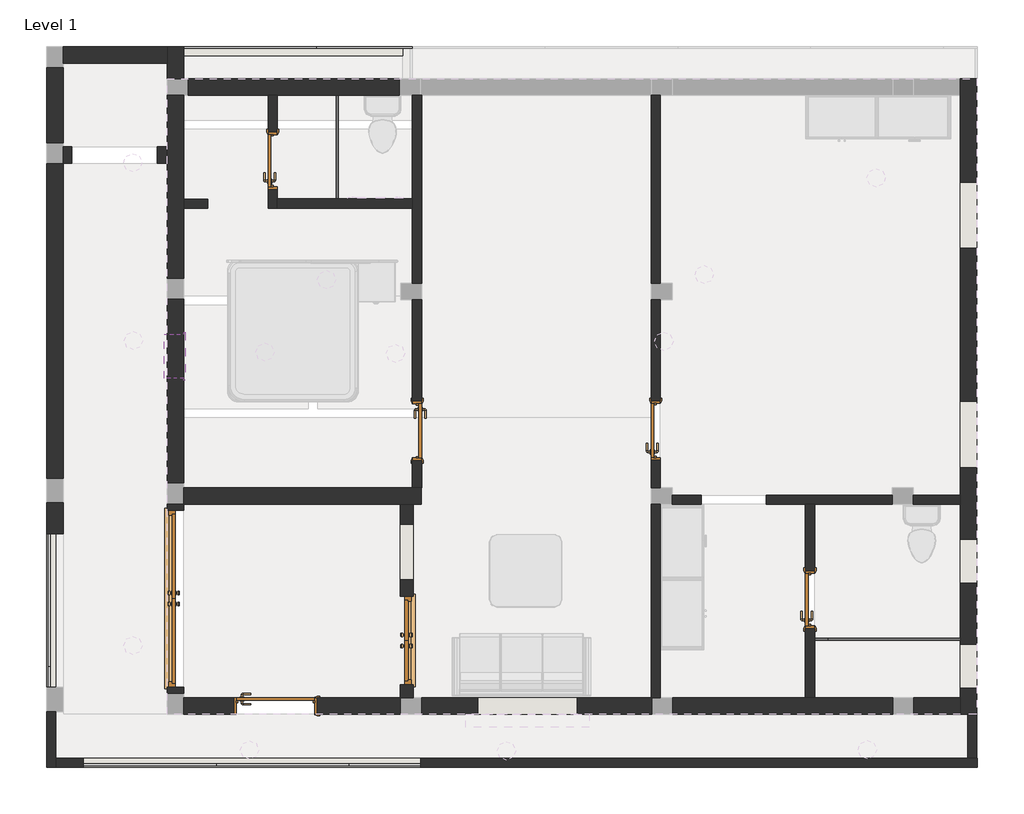
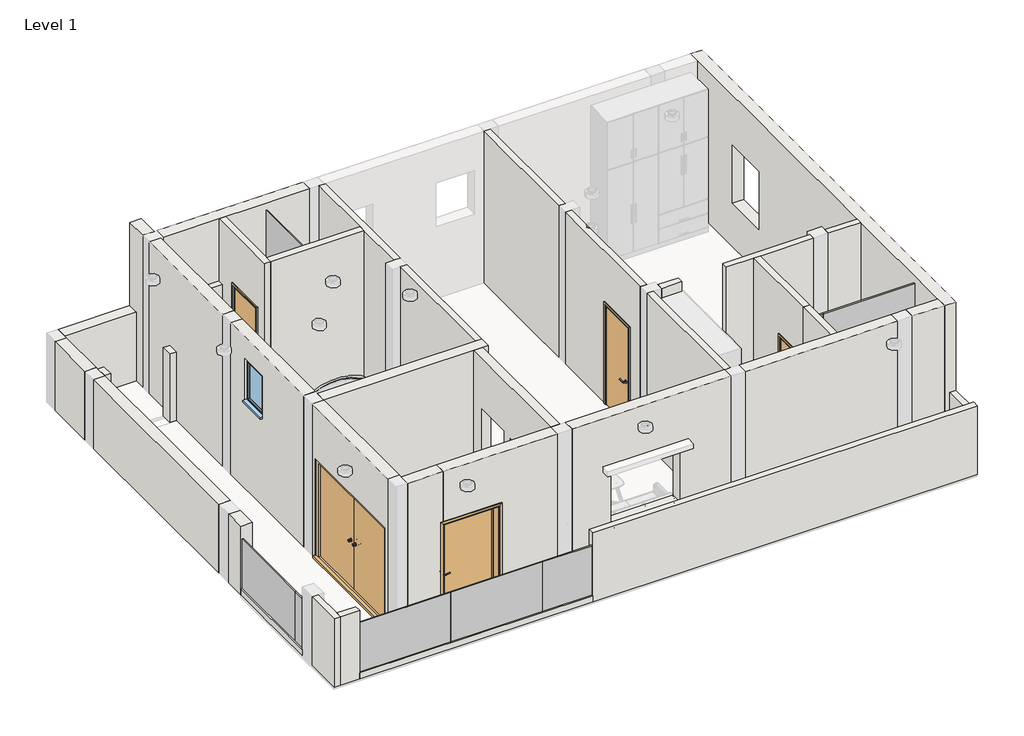
# One storey, part 1 of 2: 39 walls, 10 plates, 7 doors, 1 window.
"""IFC4 building model written with IfcOpenShell, lengths in millimetres."""

from ifc_helpers import new_model, si_unit, frame, origin, place, context, project, spatial, polyline, outline, extrude, faceted_brep, transform, mapped, element, save
from components import doors_extdbl_flush_md_0ef74d11, doors_extdbl_flush_md_2_f65acf09, doors_intsgl_d3_a25f8c6e, doors_intsgl_d4_4271d8f6, doors_intsgl_d2_d6dd0e7a, system_panel_glazed_6338a664, system_panel_glazed_e6893c60, system_panel_glazed_6661c6ea, system_panel_glazed_2d3c21f4, system_panel_glazed_3dcdd35b, system_panel_glazed_bdd68f76, system_panel_glazed_6933bc29, system_panel_glazed_1575378d, windows_sgl_plain_610x910mm_8d1346b0

model = new_model("IFC4")

# Units and contexts
model_context = context("Model", 3, world=origin())
ifc_project = project(units=[si_unit("LENGTHUNIT", "METRE", prefix="MILLI")], contexts=[model_context])

# Site, building, storey
site = spatial("IfcSite", under=ifc_project)
building = spatial("IfcBuilding", under=site)
storey = spatial("IfcBuildingStorey", under=building, Name="Level 1", Elevation=3200.4)

# Doors
placement = place(None, origin())
doors_extdbl_flush_md_shape = doors_extdbl_flush_md_0ef74d11(model_context)
element("IfcDoor", 1, ObjectType="Doors_ExtDbl_Flush : MD", at=placement, inside=storey, context=model_context, shape_type="MappedRepresentation", body=[
    mapped(doors_extdbl_flush_md_shape, transform((-11061.4858712, -2060.9296054, 3200.4), x_axis=(0.0, 1.0, 0.0), y_axis=(-1.0, 0.0, 0.0), z_axis=(0.0, 0.0, 1.0))),
])
doors_extdbl_flush_md_2_shape = doors_extdbl_flush_md_2_f65acf09(model_context)
element("IfcDoor", 2, ObjectType="Doors_ExtDbl_Flush : MD 2", at=placement, inside=storey, context=model_context, shape_type="MappedRepresentation", body=[
    mapped(doors_extdbl_flush_md_2_shape, transform((-7871.4445565, -2638.7796054, 3200.4), x_axis=(0.0, -1.0, 0.0), y_axis=(1.0, 0.0, 0.0), z_axis=(0.0, 0.0, 1.0))),
])
doors_intsgl_d3_shape = doors_intsgl_d3_a25f8c6e(model_context)
element("IfcDoor", 3, ObjectType="Doors_IntSgl : D3", at=placement, inside=storey, context=model_context, shape_type="MappedRepresentation", body=[
    mapped(doors_intsgl_d3_shape, transform((-2315.0983223, -2074.5629976, 3200.4), x_axis=(0.0, 1.0, 0.0), y_axis=(-1.0, 0.0, 0.0), z_axis=(0.0, 0.0, 1.0))),
])
element("IfcDoor", 4, ObjectType="Doors_IntSgl : D3", at=placement, inside=storey, context=model_context, shape_type="MappedRepresentation", body=[
    mapped(doors_intsgl_d3_shape, transform((-9717.6156351, 3973.7139975, 3200.4), x_axis=(0.0, 1.0, 0.0), y_axis=(-1.0, 0.0, 0.0), z_axis=(0.0, 0.0, 1.0))),
])
doors_intsgl_d4_shape = doors_intsgl_d4_4271d8f6(model_context)
element("IfcDoor", 5, ObjectType="Doors_IntSgl : D4", at=placement, inside=storey, context=model_context, shape_type="MappedRepresentation", body=[
    mapped(doors_intsgl_d4_shape, transform((-4442.6060272, 254.9952475, 3200.4), x_axis=(0.0, 1.0, 0.0), y_axis=(-1.0, 0.0, 0.0), z_axis=(0.0, 0.0, 1.0))),
])
element("IfcDoor", 6, ObjectType="Doors_IntSgl : D4", at=placement, inside=storey, context=model_context, shape_type="MappedRepresentation", body=[
    mapped(doors_intsgl_d4_shape, transform((-7729.6634981, 250.4703946, 3200.4), x_axis=(0.0, -1.0, 0.0), y_axis=(1.0, 0.0, 0.0), z_axis=(0.0, 0.0, 1.0))),
])
doors_intsgl_d2_shape = doors_intsgl_d2_d6dd0e7a(model_context)
element("IfcDoor", 7, ObjectType="Doors_IntSgl : d2", at=placement, inside=storey, context=model_context, shape_type="MappedRepresentation", body=[
    mapped(doors_intsgl_d2_shape, transform((-9681.1945565, -3540.4796054, 3200.4), x_axis=(1.0, 0.0, 0.0), y_axis=(0.0, 1.0, 0.0), z_axis=(0.0, 0.0, 1.0))),
])

# Plates
system_panel_glazed_shape = system_panel_glazed_6338a664(model_context)
element("IfcPlate", 8, ObjectType="System Panel : Glazed", at=placement, inside=storey, context=model_context, shape_type="MappedRepresentation", body=[
    mapped(system_panel_glazed_shape, transform((-10032.185871, 5496.5824405, 3200.4), x_axis=(1.0, 0.0, 0.0), y_axis=(0.0, 1.0, 0.0), z_axis=(0.0, 0.0, 1.0))),
])
system_panel_glazed_2_shape = system_panel_glazed_e6893c60(model_context)
element("IfcPlate", 9, ObjectType="System Panel : Glazed", at=placement, inside=storey, context=model_context, shape_type="MappedRepresentation", body=[
    mapped(system_panel_glazed_2_shape, transform((-8458.035871, 5496.5824405, 3200.4), x_axis=(1.0, 0.0, 0.0), y_axis=(0.0, 1.0, 0.0), z_axis=(0.0, 0.0, 1.0))),
])
system_panel_glazed_3_shape = system_panel_glazed_6661c6ea(model_context)
element("IfcPlate", 10, ObjectType="System Panel : Glazed", at=placement, inside=storey, context=model_context, shape_type="MappedRepresentation", body=[
    mapped(system_panel_glazed_3_shape, transform((-1157.4352301, -2582.5629976, 3200.4), x_axis=(-1.0, 0.0, 0.0), y_axis=(0.0, -1.0, 0.0), z_axis=(0.0, 0.0, 1.0))),
])
system_panel_glazed_4_shape = system_panel_glazed_2d3c21f4(model_context)
element("IfcPlate", 11, ObjectType="System Panel : Glazed", at=placement, inside=storey, context=model_context, shape_type="MappedRepresentation", body=[
    mapped(system_panel_glazed_4_shape, transform((-2162.0167763, -2582.5629976, 3200.4), x_axis=(-1.0, 0.0, 0.0), y_axis=(0.0, -1.0, 0.0), z_axis=(0.0, 0.0, 1.0))),
])
system_panel_glazed_5_shape = system_panel_glazed_3dcdd35b(model_context)
element("IfcPlate", 12, ObjectType="System Panel : Glazed", at=placement, inside=storey, context=model_context, shape_type="MappedRepresentation", body=[
    mapped(system_panel_glazed_5_shape, transform((-12836.0604224, -2082.0550561, 3327.4), x_axis=(0.0, -1.0, 0.0), y_axis=(1.0, 0.0, 0.0), z_axis=(0.0, 0.0, 1.0))),
])
element("IfcPlate", 13, ObjectType="System Panel : Glazed", at=placement, inside=storey, context=model_context, shape_type="MappedRepresentation", body=[
    mapped(system_panel_glazed_5_shape, transform((-11413.0604222, -4385.9896501, 3327.4), x_axis=(1.0, 0.0, 0.0), y_axis=(0.0, 1.0, 0.0), z_axis=(0.0, 0.0, 1.0))),
])
element("IfcPlate", 14, ObjectType="System Panel : Glazed", at=placement, inside=storey, context=model_context, shape_type="MappedRepresentation", body=[
    mapped(system_panel_glazed_5_shape, transform((-9583.060422, -4385.9896501, 3327.4), x_axis=(1.0, 0.0, 0.0), y_axis=(0.0, 1.0, 0.0), z_axis=(0.0, 0.0, 1.0))),
])
system_panel_glazed_6_shape = system_panel_glazed_bdd68f76(model_context)
element("IfcPlate", 15, ObjectType="System Panel : Glazed", at=placement, inside=storey, context=model_context, shape_type="MappedRepresentation", body=[
    mapped(system_panel_glazed_6_shape, transform((-8173.172826, -4385.9896501, 3327.4), x_axis=(1.0, 0.0, 0.0), y_axis=(0.0, 1.0, 0.0), z_axis=(0.0, 0.0, 1.0))),
])
system_panel_glazed_7_shape = system_panel_glazed_6933bc29(model_context)
element("IfcPlate", 16, ObjectType="System Panel : Glazed", at=placement, inside=storey, context=model_context, shape_type="MappedRepresentation", body=[
    mapped(system_panel_glazed_7_shape, transform((-12836.0604224, -3139.0723532, 3327.4), x_axis=(0.0, -1.0, 0.0), y_axis=(1.0, 0.0, 0.0), z_axis=(0.0, 0.0, 1.0))),
])
system_panel_glazed_8_shape = system_panel_glazed_1575378d(model_context)
element("IfcPlate", 17, ObjectType="System Panel : Glazed", at=placement, inside=storey, context=model_context, shape_type="MappedRepresentation", body=[
    mapped(system_panel_glazed_8_shape, transform((-8866.3134981, 4161.7783231, 3200.4), x_axis=(0.0, -1.0, 0.0), y_axis=(1.0, 0.0, 0.0), z_axis=(0.0, 0.0, 1.0))),
])

# Walls
element("IfcWall", 18, ObjectType="5\"", at=placement, inside=storey, context=model_context, shape_type="Brep", body=[
    faceted_brep([(-7926.5134981, 5546.4824405, 3200.4), (-10947.1858712, 5546.4824405, 3200.4), (-10947.1858712, 5546.4824405, 3276.6), (-7926.5134981, 5546.4824405, 3276.6), (-7926.5134981, 5419.4824405, 3200.4), (-7926.5134981, 5419.4824405, 3276.6), (-10947.1858712, 5419.4824405, 3276.6), (-10947.1858712, 5419.4824405, 3200.4), (-10947.1858712, 5545.7949405, 3200.4)], [[[0, 1, 2, 3]], [[4, 5, 6, 7]], [[1, 0, 4, 7, 8]], [[2, 1, 8, 7, 6]], [[3, 2, 6, 5]], [[0, 3, 5, 4]]]),
])
element("IfcWall", 19, ObjectType="5\"", at=placement, inside=storey, context=model_context, shape_type="Brep", body=[
    faceted_brep([(-12836.0604224, -3623.9896501, 3200.4), (-12836.0604224, -4385.9896501, 3200.4), (-12836.0604224, -4385.9896501, 4648.2), (-12836.0604224, -3623.9896501, 4648.2), (-12709.0604224, -3623.9896501, 3200.4), (-12709.0604224, -3623.9896501, 4648.2), (-12709.0604224, -4258.9896501, 4648.2), (-12709.0604224, -4385.9896501, 4648.2), (-12709.0604224, -4385.9896501, 3200.4), (-12709.0604224, -4258.9896501, 3200.4)], [[[0, 1, 2, 3]], [[4, 5, 6, 7, 8, 9]], [[1, 0, 4, 9, 8]], [[2, 1, 8, 7]], [[3, 2, 7, 6, 5]], [[0, 3, 5, 4]]]),
])
element("IfcWall", 20, ObjectType="5\"", at=placement, inside=storey, context=model_context, shape_type="Brep", body=[
    faceted_brep([(-12709.0604224, -4385.9896501, 3200.4), (-12328.0604224, -4385.9896501, 3200.4), (-12328.0604224, -4385.9896501, 3327.4), (-12328.0604224, -4385.9896501, 4648.2), (-12709.0604224, -4385.9896501, 4648.2), (-12709.0604224, -4258.9896501, 3200.4), (-12709.0604224, -4258.9896501, 4648.2), (-12328.0604224, -4258.9896501, 4648.2), (-12328.0604224, -4258.9896501, 3327.4), (-12328.0604224, -4258.9896501, 3200.4)], [[[0, 1, 2, 3, 4]], [[5, 6, 7, 8, 9]], [[1, 0, 5, 9]], [[3, 2, 1, 9, 8, 7]], [[4, 3, 7, 6]], [[0, 4, 6, 5]]]),
])
element("IfcWall", 21, ObjectType="5\"", at=placement, inside=storey, context=model_context, shape_type="Brep", body=[
    faceted_brep([(-7678.28523, -4385.9896501, 3200.4), (-7.48523, -4385.9896501, 3200.4), (-7.48523, -4385.9896501, 4648.2), (-7678.28523, -4385.9896501, 4648.2), (-7678.28523, -4385.9896501, 3327.4), (-7678.28523, -4258.9896501, 3200.4), (-7678.28523, -4258.9896501, 3327.4), (-7678.28523, -4258.9896501, 4648.2), (-7.48523, -4258.9896501, 4648.2), (-7.48523, -4258.9896501, 3200.4), (-13.83523, -4258.9896501, 3200.4), (-140.83523, -4258.9896501, 3200.4)], [[[0, 1, 2, 3, 4]], [[5, 6, 7, 8, 9, 10, 11]], [[1, 0, 5, 11, 10, 9]], [[2, 1, 9, 8]], [[3, 2, 8, 7]], [[0, 4, 3, 7, 6, 5]]]),
])
element("IfcWall", 22, ObjectType="5\"", at=placement, inside=storey, context=model_context, shape_type="SweptSolid", body=[
    extrude(outline(polyline([(-13.83523, -3654.7796054), (-13.83523, -4258.9896501), (-140.83523, -4258.9896501), (-140.83523, -3654.7796054), (-13.83523, -3654.7796054)])), frame((0.0, 0.0, 3200.4), z_axis=(0.0, 0.0, 1.0), x_axis=(1.0, 0.0, 0.0)), (0.0, 0.0, 1.0), 1333.7357837),
])
element("IfcWall", 23, ObjectType="5\"", at=placement, inside=storey, context=model_context, shape_type="SweptSolid", body=[
    extrude(outline(polyline([(-12836.0604224, -3281.0896501), (-12836.0604224, -1167.055056), (-12709.0604224, -1167.055056), (-12709.0604224, -3281.0896501), (-12836.0604224, -3281.0896501)])), frame((0.0, 0.0, 3200.4), z_axis=(0.0, 0.0, 1.0), x_axis=(1.0, 0.0, 0.0)), (0.0, 0.0, 1.0), 127.0),
])
element("IfcWall", 24, ObjectType="5\"", at=placement, inside=storey, context=model_context, shape_type="SweptSolid", body=[
    extrude(outline(polyline([(-7678.28523, -4385.9896501), (-12328.0604224, -4385.9896501), (-12328.0604224, -4258.9896501), (-7678.28523, -4258.9896501), (-7678.28523, -4385.9896501)])), frame((0.0, 0.0, 3200.4), z_axis=(0.0, 0.0, 1.0), x_axis=(1.0, 0.0, 0.0)), (0.0, 0.0, 1.0), 127.0),
])
element("IfcWall", 25, ObjectType="7\"", at=placement, inside=storey, context=model_context, shape_type="SweptSolid", body=[
    extrude(outline(polyline([(-3248.3796054, 5310.4), (-3248.3796054, 3200.4), (-3426.1796054, 3200.4), (-3426.1796054, 6400.8), (-759.1796054, 6400.8), (-759.1796054, 3200.4), (-2029.1796054, 3200.4), (-2029.1796054, 5310.4), (-3248.3796054, 5310.4)]), holes=[polyline([(-1038.5796054, 5334.0), (-1800.5796054, 5334.0), (-1800.5796054, 4114.8), (-1038.5796054, 4114.8), (-1038.5796054, 5334.0)])]), frame((-7960.3445565, 0.0, 0.0), z_axis=(1.0, 0.0, 0.0), x_axis=(0.0, 1.0, 0.0)), (0.0, 0.0, 1.0), 177.8),
])
element("IfcWall", 26, ObjectType="9\"", at=placement, inside=storey, context=model_context, shape_type="SweptSolid", body=[
    extrude(outline(polyline([(-12836.0604224, 4222.4988089), (-12836.0604224, 5253.6949405), (-12607.4604224, 5253.6949405), (-12607.4604224, 4222.4988089), (-12836.0604224, 4222.4988089)])), frame((0.0, 0.0, 3200.4), z_axis=(0.0, 0.0, 1.0), x_axis=(1.0, 0.0, 0.0)), (0.0, 0.0, 1.0), 1447.8),
])
element("IfcWall", 27, ObjectType="9\"", at=placement, inside=storey, context=model_context, shape_type="SweptSolid", body=[
    extrude(outline(polyline([(-12836.0604224, -404.5396501), (-12836.0604224, 3930.3988089), (-12607.4604224, 3930.3988089), (-12607.4604224, -404.5396501), (-12836.0604224, -404.5396501)])), frame((0.0, 0.0, 3200.4), z_axis=(0.0, 0.0, 1.0), x_axis=(1.0, 0.0, 0.0)), (0.0, 0.0, 1.0), 1447.8),
])
element("IfcWall", 28, ObjectType="9\"", at=placement, inside=storey, context=model_context, shape_type="Brep", body=[
    faceted_brep([(-12836.0604224, -743.5406999, 3200.4), (-12836.0604224, -747.4396501, 3200.4), (-12836.0604224, -1167.055056, 3200.4), (-12836.0604224, -1167.055056, 4648.2), (-12836.0604224, -743.5406999, 4648.2), (-12607.4604224, -743.5406999, 3200.4), (-12607.4604224, -743.5406999, 4648.2), (-12607.4604224, -1167.055056, 4648.2), (-12607.4604224, -1167.055056, 3200.4), (-12607.4604224, -747.4396501, 3200.4)], [[[0, 1, 2, 3, 4]], [[5, 6, 7, 8, 9]], [[2, 1, 0, 5, 9, 8]], [[3, 2, 8, 7]], [[4, 3, 7, 6]], [[0, 4, 6, 5]]]),
])
element("IfcWall", 29, ObjectType="9\"", at=placement, inside=storey, context=model_context, shape_type="SweptSolid", body=[
    extrude(outline(polyline([(6400.8, -10240.7910021), (6400.8, -10947.1858712), (3200.4, -10947.1858712), (3200.4, -10259.0445565), (5310.4, -10259.0445565), (5310.4, -10240.7910021), (6400.8, -10240.7910021)])), frame((0.0, -3654.7796054, 0.0), z_axis=(0.0, 1.0, 0.0), x_axis=(0.0, 0.0, 1.0)), (0.0, 0.0, 1.0), 228.6),
])
element("IfcWall", 30, ObjectType="9\"", at=placement, inside=storey, context=model_context, shape_type="SweptSolid", body=[
    extrude(outline(polyline([(3200.4, -7960.3445565), (6400.8, -7960.3445565), (6400.8, -10240.7910021), (5310.4, -10240.7910021), (5310.4, -9103.3445565), (3200.4, -9103.3445565), (3200.4, -7960.3445565)])), frame((0.0, -3654.7796054, 0.0), z_axis=(0.0, 1.0, 0.0), x_axis=(0.0, 0.0, 1.0)), (0.0, 0.0, 1.0), 228.6),
])
element("IfcWall", 31, ObjectType="9\"", at=placement, inside=storey, context=model_context, shape_type="SweptSolid", body=[
    extrude(outline(polyline([(3200.4, -7668.2445565), (3200.4, -4496.93523), (6400.8, -4496.93523), (6400.8, -7668.2445565), (3200.4, -7668.2445565)]), holes=[polyline([(5334.0, -6890.88523), (5334.0, -5519.28523), (4114.8, -5519.28523), (4114.8, -6890.88523), (5334.0, -6890.88523)])]), frame((0.0, -3654.7796054, 0.0), z_axis=(0.0, 1.0, 0.0), x_axis=(0.0, 0.0, 1.0)), (0.0, 0.0, 1.0), 228.6),
])
element("IfcWall", 32, ObjectType="9\"", at=placement, inside=storey, context=model_context, shape_type="SweptSolid", body=[
    extrude(outline(polyline([(-1175.88523, -3654.7796054), (-4204.83523, -3654.7796054), (-4204.83523, -3426.1796054), (-1175.88523, -3426.1796054), (-1175.88523, -3654.7796054)])), frame((0.0, 0.0, 3200.4), z_axis=(0.0, 0.0, 1.0), x_axis=(1.0, 0.0, 0.0)), (0.0, 0.0, 1.0), 3200.4),
])
element("IfcWall", 33, ObjectType="9\"", at=placement, inside=storey, context=model_context, shape_type="SweptSolid", body=[
    extrude(outline(polyline([(-242.43523, -3654.7796054), (-883.78523, -3654.7796054), (-883.78523, -3426.1796054), (-242.43523, -3426.1796054), (-242.43523, -3654.7796054)])), frame((0.0, 0.0, 3200.4), z_axis=(0.0, 0.0, 1.0), x_axis=(1.0, 0.0, 0.0)), (0.0, 0.0, 1.0), 3200.4),
])
element("IfcWall", 34, ObjectType="9\"", at=placement, inside=storey, context=model_context, shape_type="Brep", body=[
    faceted_brep([(-13.83523, -3654.7796054, 3200.4), (-13.83523, 5101.6327475, 3200.4), (-13.83523, 5101.6327475, 6400.8), (-13.83523, -3654.7796054, 6400.8), (-13.83523, -3654.7796054, 4534.1357837), (-13.83523, 2764.8327475, 5334.0), (-13.83523, 3679.2327475, 5334.0), (-13.83523, 3679.2327475, 4114.8), (-13.83523, 2764.8327475, 4114.8), (-13.83523, -257.7672525, 5334.0), (-13.83523, 656.6327475, 5334.0), (-13.83523, 656.6327475, 4114.8), (-13.83523, -257.7672525, 4114.8), (-13.83523, -2689.5796054, 4724.4), (-13.83523, -2689.5796054, 4114.8), (-13.83523, -3299.1796054, 4114.8), (-13.83523, -3299.1796054, 4724.4), (-13.83523, -1241.7796054, 4724.4), (-13.83523, -1241.7796054, 4114.8), (-13.83523, -1851.3796054, 4114.8), (-13.83523, -1851.3796054, 4724.4), (-242.43523, -3654.7796054, 3200.4), (-242.43523, -3654.7796054, 6400.8), (-242.43523, -3426.1796054, 6400.8), (-242.43523, 4873.0327475, 6400.8), (-242.43523, 5101.6327475, 6400.8), (-242.43523, 5101.6327475, 3200.4), (-242.43523, 4873.0327475, 3200.4), (-242.43523, -3426.1796054, 3200.4), (-242.43523, 2764.8327475, 5334.0), (-242.43523, 2764.8327475, 4114.8), (-242.43523, 3679.2327475, 4114.8), (-242.43523, 3679.2327475, 5334.0), (-242.43523, -257.7672525, 5334.0), (-242.43523, -257.7672525, 4114.8), (-242.43523, 656.6327475, 4114.8), (-242.43523, 656.6327475, 5334.0), (-242.43523, -2689.5796054, 4724.4), (-242.43523, -3299.1796054, 4724.4), (-242.43523, -3299.1796054, 4114.8), (-242.43523, -2689.5796054, 4114.8), (-242.43523, -1241.7796054, 4724.4), (-242.43523, -1851.3796054, 4724.4), (-242.43523, -1851.3796054, 4114.8), (-242.43523, -1241.7796054, 4114.8), (-140.83523, -3654.7796054, 3200.4)], [[[0, 1, 2, 3, 4], [5, 6, 7, 8], [9, 10, 11, 12], [13, 14, 15, 16], [17, 18, 19, 20]], [[21, 22, 23, 24, 25, 26, 27, 28], [29, 30, 31, 32], [33, 34, 35, 36], [37, 38, 39, 40], [41, 42, 43, 44]], [[1, 0, 45, 21, 28, 27, 26]], [[2, 1, 26, 25]], [[3, 2, 25, 24, 23, 22]], [[0, 4, 3, 22, 21, 45]], [[30, 29, 5, 8]], [[31, 30, 8, 7]], [[32, 31, 7, 6]], [[29, 32, 6, 5]], [[34, 33, 9, 12]], [[35, 34, 12, 11]], [[36, 35, 11, 10]], [[33, 36, 10, 9]], [[14, 13, 37, 40]], [[15, 14, 40, 39]], [[16, 15, 39, 38]], [[13, 16, 38, 37]], [[18, 17, 41, 44]], [[19, 18, 44, 43]], [[20, 19, 43, 42]], [[17, 20, 42, 41]]]),
])
element("IfcWall", 35, ObjectType="9\"", at=placement, inside=storey, context=model_context, shape_type="SweptSolid", body=[
    extrude(outline(polyline([(-11175.7858712, 5317.1949405), (-12607.4604224, 5317.1949405), (-12607.4604224, 5545.7949405), (-11175.7858712, 5545.7949405), (-11175.7858712, 5317.1949405)])), frame((0.0, 0.0, 3200.4), z_axis=(0.0, 0.0, 1.0), x_axis=(1.0, 0.0, 0.0)), (0.0, 0.0, 1.0), 1447.8),
])
element("IfcWall", 36, ObjectType="9\"", at=placement, inside=storey, context=model_context, shape_type="Brep", body=[
    faceted_brep([(-11175.7858712, 5545.7949405, 3200.4), (-11175.7858712, 5317.1949405, 3200.4), (-11175.7858712, 5105.4926487, 3200.4), (-11175.7858712, 5105.4926487, 6400.8), (-11175.7858712, 5545.7949405, 6400.8), (-11175.7858712, 5545.7949405, 4648.2), (-10947.1858712, 5545.7949405, 3200.4), (-10947.1858712, 5545.7949405, 6400.8), (-10947.1858712, 5105.4926487, 6400.8), (-10947.1858712, 5105.4926487, 3200.4), (-10947.1858712, 5419.4824405, 3200.4)], [[[0, 1, 2, 3, 4, 5]], [[6, 7, 8, 9, 10]], [[2, 1, 0, 6, 10, 9]], [[3, 2, 9, 8]], [[4, 3, 8, 7]], [[0, 5, 4, 7, 6]]]),
])
element("IfcWall", 37, ObjectType="9\"", at=placement, inside=storey, context=model_context, shape_type="Brep", body=[
    faceted_brep([(-11175.7858712, 4876.8926487, 3200.4), (-11175.7858712, 4168.5238089, 3200.4), (-11175.7858712, 3939.9238089, 3200.4), (-11175.7858712, 2353.0673305, 3200.4), (-11175.7858712, 2353.0673305, 6400.8), (-11175.7858712, 4876.8926487, 6400.8), (-10947.1858712, 4876.8926487, 3200.4), (-10947.1858712, 4876.8926487, 6400.8), (-10947.1858712, 2353.0673305, 6400.8), (-10947.1858712, 2353.0673305, 3200.4)], [[[0, 1, 2, 3, 4, 5]], [[6, 7, 8, 9]], [[3, 2, 1, 0, 6, 9]], [[4, 3, 9, 8]], [[5, 4, 8, 7]], [[0, 5, 7, 6]]]),
])
element("IfcWall", 38, ObjectType="9\"", at=placement, inside=storey, context=model_context, shape_type="SweptSolid", body=[
    extrude(outline(polyline([(2065.5455124, 3200.4), (-467.0796054, 3200.4), (-467.0796054, 6400.8), (2065.5455124, 6400.8), (2065.5455124, 3200.4)]), holes=[polyline([(973.3455124, 5939.2), (973.3455124, 5029.2), (1582.9455124, 5029.2), (1582.9455124, 5939.2), (973.3455124, 5939.2)])]), frame((-11175.7858712, 0.0, 0.0), z_axis=(1.0, 0.0, 0.0), x_axis=(0.0, 1.0, 0.0)), (0.0, 0.0, 1.0), 228.6),
])
element("IfcWall", 39, ObjectType="9\"", at=placement, inside=storey, context=model_context, shape_type="SweptSolid", body=[
    extrude(outline(polyline([(-759.1796054, 3200.4), (-841.7296054, 3200.4), (-841.7296054, 5310.4), (-3280.1296054, 5310.4), (-3280.1296054, 3200.4), (-3362.6796054, 3200.4), (-3362.6796054, 6400.8), (-759.1796054, 6400.8), (-759.1796054, 3200.4)])), frame((-11175.7858712, 0.0, 0.0), z_axis=(1.0, 0.0, 0.0), x_axis=(0.0, 1.0, 0.0)), (0.0, 0.0, 1.0), 228.6),
])
element("IfcWall", 40, ObjectType="9\"", at=placement, inside=storey, context=model_context, shape_type="SweptSolid", body=[
    extrude(outline(polyline([(-12486.8104224, 3939.9238089), (-12607.4604224, 3939.9238089), (-12607.4604224, 4168.5238089), (-12486.8104224, 4168.5238089), (-12486.8104224, 3939.9238089)])), frame((0.0, 0.0, 3200.4), z_axis=(0.0, 0.0, 1.0), x_axis=(1.0, 0.0, 0.0)), (0.0, 0.0, 1.0), 1447.8),
])
element("IfcWall", 41, ObjectType="9\"", at=placement, inside=storey, context=model_context, shape_type="SweptSolid", body=[
    extrude(outline(polyline([(-11175.7858712, 3939.9238089), (-11308.4687707, 3939.9238089), (-11308.4687707, 4168.5238089), (-11175.7858712, 4168.5238089), (-11175.7858712, 3939.9238089)])), frame((0.0, 0.0, 3200.4), z_axis=(0.0, 0.0, 1.0), x_axis=(1.0, 0.0, 0.0)), (0.0, 0.0, 1.0), 1447.8),
])
element("IfcWall", 42, ObjectType="brick 5\"", at=placement, inside=storey, context=model_context, shape_type="Brep", body=[
    faceted_brep([(-7793.1634981, 4873.0327475, 3200.4), (-7793.1634981, 3446.6639975, 3200.4), (-7793.1634981, 3319.6639975, 3200.4), (-7793.1634981, 2285.4077475, 3200.4), (-7793.1634981, 2285.4077475, 6400.8), (-7793.1634981, 3319.6639975, 6400.8), (-7793.1634981, 3446.6639975, 6400.8), (-7793.1634981, 4873.0327475, 6400.8), (-7666.1634981, 4873.0327475, 3200.4), (-7666.1634981, 4873.0327475, 6400.8), (-7666.1634981, 2285.4077475, 6400.8), (-7666.1634981, 2285.4077475, 3200.4), (-7680.825513, 4873.0327475, 3200.4), (-7680.825513, 4873.0327475, 6400.8)], [[[0, 1, 2, 3, 4, 5, 6, 7]], [[8, 9, 10, 11]], [[3, 2, 1, 0, 12, 8, 11]], [[4, 3, 11, 10]], [[7, 6, 5, 4, 10, 9, 13]], [[0, 7, 13, 9, 8, 12]]]),
])
element("IfcWall", 43, ObjectType="brick 5\"", at=placement, inside=storey, context=model_context, shape_type="SweptSolid", body=[
    extrude(outline(polyline([(-4506.1060272, 2285.4077475), (-4506.1060272, 4873.0327475), (-4379.1060272, 4873.0327475), (-4379.1060272, 2285.4077475), (-4506.1060272, 2285.4077475)])), frame((0.0, 0.0, 3200.4), z_axis=(0.0, 0.0, 1.0), x_axis=(1.0, 0.0, 0.0)), (0.0, 0.0, 1.0), 3200.4),
])
element("IfcWall", 44, ObjectType="brick 5\"", at=placement, inside=storey, context=model_context, shape_type="SweptSolid", body=[
    extrude(outline(polyline([(-535.5797525, 3200.4), (-535.5797525, 6400.8), (2056.8077475, 6400.8), (2056.8077475, 3200.4), (667.7452475, 3200.4), (667.7452475, 5310.4), (-157.7547525, 5310.4), (-157.7547525, 3200.4), (-535.5797525, 3200.4)])), frame((-4506.1060272, 0.0, 0.0), z_axis=(1.0, 0.0, 0.0), x_axis=(0.0, 1.0, 0.0)), (0.0, 0.0, 1.0), 127.0),
])
element("IfcWall", 45, ObjectType="brick 5\"", at=placement, inside=storey, context=model_context, shape_type="SweptSolid", body=[
    extrude(outline(polyline([(-4506.1060272, -3426.1796054), (-4506.1060272, -764.1797525), (-4379.1060272, -764.1797525), (-4379.1060272, -3426.1796054), (-4506.1060272, -3426.1796054)])), frame((0.0, 0.0, 3200.4), z_axis=(0.0, 0.0, 1.0), x_axis=(1.0, 0.0, 0.0)), (0.0, 0.0, 1.0), 3200.4),
])
element("IfcWall", 46, ObjectType="brick 5\"", at=placement, inside=storey, context=model_context, shape_type="SweptSolid", body=[
    extrude(outline(polyline([(-3813.9560272, -764.1797525), (-4214.0060272, -764.1797525), (-4214.0060272, -637.1797525), (-3813.9560272, -637.1797525), (-3813.9560272, -764.1797525)])), frame((0.0, 0.0, 3200.4), z_axis=(0.0, 0.0, 1.0), x_axis=(1.0, 0.0, 0.0)), (0.0, 0.0, 1.0), 3200.4),
])
element("IfcWall", 47, ObjectType="brick 5\"", at=placement, inside=storey, context=model_context, shape_type="Brep", body=[
    faceted_brep([(-2920.6153893, -764.1797525, 3200.4), (-2378.5983223, -764.1797525, 3200.4), (-2251.5983223, -764.1797525, 3200.4), (-1182.23523, -764.1797525, 3200.4), (-1182.23523, -764.1797525, 6400.8), (-2251.5983223, -764.1797525, 6400.8), (-2378.5983223, -764.1797525, 6400.8), (-2920.6153893, -764.1797525, 6400.8), (-2920.6153893, -637.1797525, 3200.4), (-2920.6153893, -637.1797525, 6400.8), (-1182.23523, -637.1797525, 6400.8), (-1182.23523, -637.1797525, 3200.4)], [[[0, 1, 2, 3, 4, 5, 6, 7]], [[8, 9, 10, 11]], [[3, 2, 1, 0, 8, 11]], [[4, 3, 11, 10]], [[7, 6, 5, 4, 10, 9]], [[0, 7, 9, 8]]]),
])
element("IfcWall", 48, ObjectType="brick 5\"", at=placement, inside=storey, context=model_context, shape_type="SweptSolid", body=[
    extrude(outline(polyline([(-242.43523, -764.1797525), (-890.13523, -764.1797525), (-890.13523, -637.1797525), (-242.43523, -637.1797525), (-242.43523, -764.1797525)])), frame((0.0, 0.0, 3200.4), z_axis=(0.0, 0.0, 1.0), x_axis=(1.0, 0.0, 0.0)), (0.0, 0.0, 1.0), 3200.4),
])
element("IfcWall", 49, ObjectType="brick 5\"", at=placement, inside=storey, context=model_context, shape_type="SweptSolid", body=[
    extrude(outline(polyline([(-2474.6129976, 6400.8), (-764.1797525, 6400.8), (-764.1797525, 3200.4), (-1674.5129976, 3200.4), (-1674.5129976, 5310.4), (-2474.6129976, 5310.4), (-2474.6129976, 6400.8)])), frame((-2378.5983223, 0.0, 0.0), z_axis=(1.0, 0.0, 0.0), x_axis=(0.0, 1.0, 0.0)), (0.0, 0.0, 1.0), 127.0),
])
element("IfcWall", 50, ObjectType="brick 5\"", at=placement, inside=storey, context=model_context, shape_type="SweptSolid", body=[
    extrude(outline(polyline([(-2378.5983223, -3426.1796054), (-2378.5983223, -2474.6129976), (-2251.5983223, -2474.6129976), (-2251.5983223, -3426.1796054), (-2378.5983223, -3426.1796054)])), frame((0.0, 0.0, 3200.4), z_axis=(0.0, 0.0, 1.0), x_axis=(1.0, 0.0, 0.0)), (0.0, 0.0, 1.0), 3200.4),
])
element("IfcWall", 51, ObjectType="brick 5\"", at=placement, inside=storey, context=model_context, shape_type="SweptSolid", body=[
    extrude(outline(polyline([(-530.5796054, 3200.4), (-530.5796054, 6400.8), (2056.8077475, 6400.8), (2056.8077475, 3200.4), (663.2203946, 3200.4), (663.2203946, 5310.4), (-162.2796054, 5310.4), (-162.2796054, 3200.4), (-530.5796054, 3200.4)])), frame((-7793.1634981, 0.0, 0.0), z_axis=(1.0, 0.0, 0.0), x_axis=(0.0, 1.0, 0.0)), (0.0, 0.0, 1.0), 127.0),
])
element("IfcWall", 52, ObjectType="brick 5\"", at=placement, inside=storey, context=model_context, shape_type="SweptSolid", body=[
    extrude(outline(polyline([(-9654.1156351, 3446.6639975), (-7793.1634981, 3446.6639975), (-7793.1634981, 3319.6639975), (-9654.1156351, 3319.6639975), (-9654.1156351, 3446.6639975)])), frame((0.0, 0.0, 3200.4), z_axis=(0.0, 0.0, 1.0), x_axis=(1.0, 0.0, 0.0)), (0.0, 0.0, 1.0), 3200.4),
])
element("IfcWall", 53, ObjectType="brick 5\"", at=placement, inside=storey, context=model_context, shape_type="SweptSolid", body=[
    extrude(outline(polyline([(3319.6639975, 3200.4), (3319.6639975, 6400.8), (4873.0327475, 6400.8), (4873.0327475, 3200.4), (4373.7639975, 3200.4), (4373.7639975, 5310.4), (3573.6639975, 5310.4), (3573.6639975, 3200.4), (3319.6639975, 3200.4)])), frame((-9781.1156351, 0.0, 0.0), z_axis=(1.0, 0.0, 0.0), x_axis=(0.0, 1.0, 0.0)), (0.0, 0.0, 1.0), 127.0),
])
element("IfcWall", 54, ObjectType="brick 5\"", at=placement, inside=storey, context=model_context, shape_type="SweptSolid", body=[
    extrude(outline(polyline([(-10616.9858712, 3318.2673305), (-10947.1858712, 3318.2673305), (-10947.1858712, 3445.2673305), (-10616.9858712, 3445.2673305), (-10616.9858712, 3318.2673305)])), frame((0.0, 0.0, 3200.4), z_axis=(0.0, 0.0, 1.0), x_axis=(1.0, 0.0, 0.0)), (0.0, 0.0, 1.0), 3048.0),
])
element("IfcWall", 55, ObjectType="brick 9\"", at=placement, inside=storey, context=model_context, shape_type="SweptSolid", body=[
    extrude(outline(polyline([(-7670.5858712, -759.1796054), (-10947.1858712, -759.1796054), (-10947.1858712, -530.5796054), (-7670.5858712, -530.5796054), (-7670.5858712, -759.1796054)])), frame((0.0, 0.0, 3200.4), z_axis=(0.0, 0.0, 1.0), x_axis=(1.0, 0.0, 0.0)), (0.0, 0.0, 1.0), 3200.4),
])
element("IfcWall", 56, ObjectType="brick 9\"", at=placement, inside=storey, context=model_context, shape_type="SweptSolid", body=[
    extrude(outline(polyline([(-10883.6959332, 5105.4926487), (-7972.925513, 5105.4926487), (-7972.925513, 4876.8926487), (-10883.6959332, 4876.8926487), (-10883.6959332, 5105.4926487)])), frame((0.0, 0.0, 3200.4), z_axis=(0.0, 0.0, 1.0), x_axis=(1.0, 0.0, 0.0)), (0.0, 0.0, 1.0), 3200.4),
])

# Window
windows_sgl_plain_610x910mm_shape = windows_sgl_plain_610x910mm_8d1346b0(model_context)
element("IfcWindow", 57, ObjectType="Windows_Sgl_Plain : 610x910mm", at=placement, inside=storey, context=model_context, shape_type="MappedRepresentation", body=[
    mapped(windows_sgl_plain_610x910mm_shape, transform((-11053.0293033, 1278.1455124, 3829.2), x_axis=(0.0, 1.0, 0.0), y_axis=(-1.0, 0.0, 0.0), z_axis=(0.0, 0.0, 1.0))),
])

save(model, "model.ifc")

# Revit data of these elements
# Type "Doors_ExtDbl_Flush : MD"
#   Type Mark = "47"
#   Type Comments = "External Double"
#   Operation = "DoubleDoorSingleSwing"
#   Keynote = "L20"
#   Analytic Construction = "Metal"
#   Wrap Layers (Ext) from Ext = 0' - 4.03543"
#   Wrap Layers (Int) from Ext = 0' - 6.98819"
#   Thickness = 0' - 1.73228"
#   Rough Width = 8' - 0"
#   Rough Height = 6' - 11.07087"
#   O/A Frame Width = 0' - 2.51969"
#   Heat Transfer Coefficient (U) = 3.7021 W/(m²·K)
#   Handle Z Distance = 3' - 5.33858"
#   FrameWidth = 0' - 1.65354"
#   FrameOffset - External = 0' - 0.98425"
#   FrameDepth = 0' - 3.50394"
#   Door Panel Width = 3' - 9.91339"
#   Door Panel Thickness = 0' - 1.73228"
#   Door Panel Height = 6' - 6.74016"
#   Cill Thickness = 0' - 2.14567"
#   Cill Projection = 0' - 1.1811"
#   Handle X Distance = 0' - 2.95276"
#   Height = 6' - 11.07087"
#   Structural Tolerance = 0' - 0.25591"
#   Tolerance = 0' - 0.11811"
#   Undercut = 0' - 0.15748"
#   Width = 8' - 0"
#   Cill Extension = 0' - 0.98425"
#   Cavity Closer Width = 0' - 1.9685"
#   Cavity Closer Offset from Ext = 0' - 4.03543"
#   Cavity Closer Depth = 0' - 3.34646"
#   Vis - Ironmongery = yes
#   Vis - Cavity Closers = yes
#   Function = 1
#   Material Door = Door - Panel
#   Material Frame = Door - Frame/Mullion
#   Material Ironmongery = Door - Handle
#   Visual Light Transmittance = 0
#   Thermal Resistance (R) = 0
#   Solar Heat Gain Coefficient = 0
#   Wall Closure = (empty or 0)
# Type "Doors_ExtDbl_Flush : MD 2"
#   Type Mark = "51"
#   Type Comments = "External Double"
#   Operation = "DoubleDoorSingleSwing"
#   Keynote = "L20"
#   Analytic Construction = "Metal"
#   Wrap Layers (Ext) from Ext = 0' - 4.03543"
#   Wrap Layers (Int) from Ext = 0' - 6.98819"
#   Thickness = 0' - 1.73228"
#   Rough Width = 4' - 0"
#   Rough Height = 6' - 11.07087"
#   O/A Frame Width = 0' - 2.51969"
#   Heat Transfer Coefficient (U) = 3.7021 W/(m²·K)
#   Handle Z Distance = 3' - 5.33858"
#   FrameWidth = 0' - 1.65354"
#   FrameOffset - External = 0' - 0.98425"
#   FrameDepth = 0' - 3.50394"
#   Door Panel Width = 1' - 9.91339"
#   Door Panel Thickness = 0' - 1.73228"
#   Door Panel Height = 6' - 6.74016"
#   Cill Thickness = 0' - 2.14567"
#   Cill Projection = 0' - 1.1811"
#   Handle X Distance = 0' - 2.95276"
#   Height = 6' - 11.07087"
#   Structural Tolerance = 0' - 0.25591"
#   Tolerance = 0' - 0.11811"
#   Undercut = 0' - 0.15748"
#   Width = 4' - 0"
#   Cill Extension = 0' - 0.98425"
#   Cavity Closer Width = 0' - 1.9685"
#   Cavity Closer Offset from Ext = 0' - 4.03543"
#   Cavity Closer Depth = 0' - 3.34646"
#   Vis - Ironmongery = yes
#   Vis - Cavity Closers = yes
#   Function = 1
#   Material Door = Door - Panel
#   Material Frame = Door - Frame/Mullion
#   Material Ironmongery = Door - Handle
#   Visual Light Transmittance = 0
#   Thermal Resistance (R) = 0
#   Solar Heat Gain Coefficient = 0
#   Wall Closure = (empty or 0)
# Type "Doors_IntSgl : D3"
#   Type Mark = "49"
#   Type Comments = "Internal Single"
#   Operation = "SingleSwingRight"
#   Manufacturer = "Revit"
#   Keynote = "L20"
#   Description = "Internal Single Door"
#   Analytic Construction = "Metal"
#   UnderCut = 0' - 0.31496"
#   Tolerance = 0' - 0.07874"
#   Thickness = 0' - 1.49606"
#   Thermal Resistance (R) = 0.270117 (m²·K)/W
#   Structural Tolerance = 0' - 0.31496"
#   StopDepth = 0' - 1.25984"
#   Stop Thickness = 0' - 0.74803"
#   Rough Width = 2' - 7 1/2"
#   Rough Height = 6' - 11.07087"
#   Height to Top Lock Rail = 3' - 3.37008"
#   Heat Transfer Coefficient (U) = 3.7021 W/(m²·K)
#   Handle Z Distance = 2' - 11.43307"
#   Handle X Distance = 0' - 2.95276"
#   Frame Thickness = 0' - 1.25984"
#   Door Panel Width = 2' - 4.19291"
#   Door Panel Thickness = 0' - 1.49606"
#   Door Panel Offset = 0' - 0"
#   Height = 6' - 11.07087"
#   Width = 2' - 7 1/2"
#   Door Panel Height = 6' - 9.10236"
#   Architrave Setback = 0' - 0.19685"
#   Vis - Ironmongery = yes
#   Material Ironmongery = Door - Handle
#   Material Frame = Door - Frame/Mullion (1)
#   Material Door = Door - Panel
#   Material Architrave = Door - Architrave
#   Visual Light Transmittance = 0
#   Solar Heat Gain Coefficient = 0
#   Function = (empty or 0)
#   Wall Closure = (empty or 0)
# Type "Doors_IntSgl : D4"
#   Type Mark = "50"
#   Type Comments = "Internal Single"
#   Operation = "SingleSwingRight"
#   Manufacturer = "Revit"
#   Keynote = "L20"
#   Description = "Internal Single Door"
#   Analytic Construction = "Metal"
#   UnderCut = 0' - 0.31496"
#   Tolerance = 0' - 0.07874"
#   Thickness = 0' - 1.49606"
#   Thermal Resistance (R) = 0.270117 (m²·K)/W
#   Structural Tolerance = 0' - 0.31496"
#   StopDepth = 0' - 1.25984"
#   Stop Thickness = 0' - 0.74803"
#   Rough Width = 2' - 8 1/2"
#   Rough Height = 6' - 11.07087"
#   Height to Top Lock Rail = 3' - 3.37008"
#   Heat Transfer Coefficient (U) = 3.7021 W/(m²·K)
#   Handle Z Distance = 2' - 11.43307"
#   Handle X Distance = 0' - 2.95276"
#   Frame Thickness = 0' - 1.25984"
#   Door Panel Width = 2' - 5.19291"
#   Door Panel Thickness = 0' - 1.49606"
#   Door Panel Offset = 0' - 0"
#   Height = 6' - 11.07087"
#   Width = 2' - 8 1/2"
#   Door Panel Height = 6' - 9.10236"
#   Architrave Setback = 0' - 0.19685"
#   Vis - Ironmongery = yes
#   Material Ironmongery = Door - Handle
#   Material Frame = Door - Frame/Mullion (1)
#   Material Door = Door - Panel
#   Material Architrave = Door - Architrave
#   Visual Light Transmittance = 0
#   Solar Heat Gain Coefficient = 0
#   Function = (empty or 0)
#   Wall Closure = (empty or 0)
# Type "Doors_IntSgl : d2"
#   Type Mark = "48"
#   Type Comments = "Internal Single"
#   Operation = "SingleSwingRight"
#   Manufacturer = "Revit"
#   Keynote = "L20"
#   Description = "Internal Single Door"
#   Analytic Construction = "Metal"
#   UnderCut = 0' - 0.31496"
#   Tolerance = 0' - 0.07874"
#   Thickness = 0' - 1.49606"
#   Thermal Resistance (R) = 0.270117 (m²·K)/W
#   Structural Tolerance = 0' - 0.31496"
#   StopDepth = 0' - 1.25984"
#   Stop Thickness = 0' - 0.74803"
#   Rough Width = 3' - 9 1/2"
#   Rough Height = 6' - 11.07087"
#   Height to Top Lock Rail = 3' - 3.37008"
#   Heat Transfer Coefficient (U) = 3.7021 W/(m²·K)
#   Handle Z Distance = 2' - 11.43307"
#   Handle X Distance = 0' - 2.95276"
#   Frame Thickness = 0' - 1.25984"
#   Door Panel Width = 3' - 6.19291"
#   Door Panel Thickness = 0' - 1.49606"
#   Door Panel Offset = 0' - 0"
#   Height = 6' - 11.07087"
#   Width = 3' - 9 1/2"
#   Door Panel Height = 6' - 9.10236"
#   Architrave Setback = 0' - 0.19685"
#   Vis - Ironmongery = yes
#   Material Ironmongery = Door - Handle
#   Material Frame = Door - Frame/Mullion (1)
#   Material Door = Door - Panel
#   Material Architrave = Door - Architrave
#   Visual Light Transmittance = 0
#   Solar Heat Gain Coefficient = 0
#   Function = (empty or 0)
#   Wall Closure = (empty or 0)
# Type "System Panel : Glazed"
#   Keynote = "H11"
#   Construction Type Id = "GSP4R"
#   Analytic Construction = "1/8 in Pilkington single glazing"
#   Visual Light Transmittance = 0.9
#   Solar Heat Gain Coefficient = 0.86
#   Heat Transfer Coefficient (U) = 6.7069 W/(m²·K)
#   Define Thermal Properties by = 1
# Type "5\""
#   Keynote = "F10"
#   Layers, outside or top first: 0' - 5" "Concrete" (function 1)
# Type "7\""
#   Keynote = "F10"
#   Layers, outside or top first: 0' - 7" "Brick, Engineering" (function 1)
# Type "9\""
#   Keynote = "F10"
#   Layers, outside or top first: 0' - 9" "Concrete" (function 1)
# Type "brick 5\""
#   Keynote = "F10"
#   Layers, outside or top first: 0' - 5" "Brick, Engineering" (function 1)
# Type "brick 9\""
#   Keynote = "F10"
#   Layers, outside or top first: 0' - 9" "Brick, Engineering" (function 1)
# Type "Windows_Sgl_Plain : 610x910mm"
#   Type Mark = "44"
#   Operation = "SinglePanel"
#   Construction Type Id = "SGL"
#   Manufacturer = "Revit"
#   Keynote = "L10"
#   Analytic Construction = "Large single-glazed windows"
#   Wrap Layers (Ext) from Ext = 0' - 4.03543"
#   Wrap Layers (Int) from Ext = 0' - 6.98819"
#   Window Board Projection = 0' - 0.98425"
#   Window Board Extension = 0' - 0.98425"
#   Visual Light Transmittance = 0.9
#   Solar Heat Gain Coefficient = 0.86
#   Rough Width = 2' - 0"
#   Rough Height = 2' - 11.82677"
#   Height = 2' - 11.82677"
#   Width = 2' - 0"
#   Heat Transfer Coefficient (U) = 5.5617 W/(m²·K)
#   Glazing Thickness = 0' - 0.94488"
#   FrameOffset - External = 0' - 1.9685"
#   Frame Depth = 0' - 2.55906"
#   Default Head Height = 6' - 11.07087"
#   Cill Depth = 0' - 3.44488"
#   Cavity Closer Width = 0' - 1.9685"
#   Cavity Closer Offset from Ext = 0' - 4.03543"
#   Cavity Closer Depth = 0' - 3.34646"
#   Define Thermal Properties by = 1
#   Vis - Cavity Closers = yes
#   Define Thermal Properties by = 1
#   Material Trim = Window Frame
#   Material Glass = Glass
#   Material Frame = Window Frame
#   Wall Closure = (empty or 0)
# Element 1 (IfcDoor, "Doors_ExtDbl_Flush : MD")
#   Phase Created = New Construction
#   Materials on its faces: "Door - Handle", "Door - Frame/Mullion", "Door - Panel"
# Element 2 (IfcDoor, "Doors_ExtDbl_Flush : MD 2")
#   Phase Created = New Construction
#   Materials on its faces: "Door - Handle", "Door - Frame/Mullion", "Door - Panel"
# Elements 3, 4 (IfcDoor, "Doors_IntSgl : D3")
#   Phase Created = New Construction
#   Materials on its faces: "Door - Architrave", "Door - Handle", "Door - Frame/Mullion (1)", "Door - Panel"
# Elements 5, 6 (IfcDoor, "Doors_IntSgl : D4")
#   Phase Created = New Construction
#   Materials on its faces: "Door - Architrave", "Door - Handle", "Door - Frame/Mullion (1)", "Door - Panel"
# Element 7 (IfcDoor, "Doors_IntSgl : d2")
#   Phase Created = New Construction
#   Materials on its faces: "Door - Architrave", "Door - Handle", "Door - Frame/Mullion (1)", "Door - Panel"
# Elements 8, 9, 10, 11, 12, 13, 14, 15, 16, 17 (IfcPlate, "System Panel : Glazed")
#   Phase Created = New Construction
#   Materials on its faces: "Glass"
# Element 18 (IfcWall, "5\"")
#   Top Offset = 0' - 0"
#   Base Offset = 0' - 0"
#   Unconnected Height = 0' - 3"
#   wall height = 0' - 3"
#   Phase Created = New Construction
#   Base Constraint = Level 1
#   Materials on its faces: "Concrete", "Gypsum Wall Board"
# Elements 19, 20 (IfcWall, "5\"")
#   Top Offset = -5' - 9"
#   Base Offset = 0' - 0"
#   wall height = 4' - 9"
#   Phase Created = New Construction
#   Base Constraint = Level 1
#   Top Constraint = Level 2
#   Materials on its faces: "Liquid - White Wine", "Concrete"
# Element 21 (IfcWall, "5\"")
#   Top Offset = -5' - 9"
#   Base Offset = 0' - 0"
#   wall height = 4' - 9"
#   Phase Created = New Construction
#   Base Constraint = Level 1
#   Top Constraint = Level 2
#   Materials on its faces: "Concrete", "Liquid - White Wine", "new"
# Element 22 (IfcWall, "5\"")
#   Top Offset = -6' - 1.49072"
#   Base Offset = 0' - 0"
#   wall height = 4' - 4.50928"
#   Phase Created = New Construction
#   Base Constraint = Level 1
#   Top Constraint = Level 2
#   Materials on its faces: "Concrete"
# Elements 23, 24 (IfcWall, "5\"")
#   Top Offset = 0' - 0"
#   Base Offset = 0' - 0"
#   Unconnected Height = 0' - 5"
#   wall height = 0' - 5"
#   Phase Created = New Construction
#   Base Constraint = Level 1
#   Materials on its faces: "Concrete", "Liquid - White Wine"
# Element 25 (IfcWall, "7\"")
#   Top Offset = 0' - 0"
#   Base Offset = 0' - 0"
#   wall height = 10' - 6"
#   Phase Created = New Construction
#   Base Constraint = Level 1
#   Top Constraint = Level 2
#   Materials on its faces: "Brick, Engineering"
# Element 26 (IfcWall, "9\"")
#   Top Offset = -5' - 9"
#   Base Offset = 0' - 0"
#   wall height = 4' - 9"
#   Phase Created = New Construction
#   Base Constraint = Level 1
#   Top Constraint = Level 2
#   Materials on its faces: "Concrete", "Gypsum Wall Board"
# Elements 27, 35, 40 (IfcWall, "9\"")
#   Top Offset = -5' - 9"
#   Base Offset = 0' - 0"
#   wall height = 4' - 9"
#   Phase Created = New Construction
#   Base Constraint = Level 1
#   Top Constraint = Level 2
#   Materials on its faces: "Gypsum Wall Board", "Concrete"
# Element 28 (IfcWall, "9\"")
#   Top Offset = -5' - 9"
#   Base Offset = 0' - 0"
#   wall height = 4' - 9"
#   Phase Created = New Construction
#   Base Constraint = Level 1
#   Top Constraint = Level 2
#   Materials on its faces: "Liquid - White Wine", "Concrete"
# Elements 29, 39 (IfcWall, "9\"")
#   Top Offset = 0' - 0"
#   Base Offset = 0' - 0"
#   wall height = 10' - 6"
#   Phase Created = New Construction
#   Base Constraint = Level 1
#   Top Constraint = Level 2
#   Materials on its faces: "Concrete", "new"
# Elements 30, 31, 32, 33, 34, 36, 37, 38 (IfcWall, "9\"")
#   Top Offset = 0' - 0"
#   Base Offset = 0' - 0"
#   wall height = 10' - 6"
#   Phase Created = New Construction
#   Base Constraint = Level 1
#   Top Constraint = Level 2
#   Materials on its faces: "Concrete", "Gypsum Wall Board"
# Element 41 (IfcWall, "9\"")
#   Top Offset = -5' - 9"
#   Base Offset = 0' - 0"
#   wall height = 4' - 9"
#   Phase Created = New Construction
#   Base Constraint = Level 1
#   Top Constraint = Level 2
#   Materials on its faces: "Concrete"
# Elements 42, 43, 44, 45, 46, 47, 48, 49, 50, 51, 52, 53 (IfcWall, "brick 5\"")
#   Top Offset = 0' - 0"
#   Base Offset = 0' - 0"
#   wall height = 10' - 6"
#   Phase Created = New Construction
#   Base Constraint = Level 1
#   Top Constraint = Level 2
#   Materials on its faces: "Brick, Engineering"
# Element 54 (IfcWall, "brick 5\"")
#   Top Offset = 0' - 0"
#   Base Offset = 0' - 0"
#   Unconnected Height = 10' - 0"
#   wall height = 10' - 0"
#   Phase Created = New Construction
#   Base Constraint = Level 1
#   Materials on its faces: "Brick, Engineering"
# Elements 55, 56 (IfcWall, "brick 9\"")
#   Top Offset = 0' - 0"
#   Base Offset = 0' - 0"
#   wall height = 10' - 6"
#   Phase Created = New Construction
#   Base Constraint = Level 1
#   Top Constraint = Level 2
#   Materials on its faces: "Brick, Engineering"
# Element 57 (IfcWindow, "Windows_Sgl_Plain : 610x910mm")
#   Mark = "9"
#   Phase Created = New Construction
#   Materials on its faces: "Window Frame", "Glass"
# Materials
#   "Door - Panel": class "Wood", colour RGB 210 159 95, transparency 0, Keynote = "L20", Cost = 0
#   "Door - Frame/Mullion": class "Wood", colour RGB 212 179 113, transparency 0, Keynote = "L20", Cost = 0
#   "Door - Handle": colour RGB 0 0 0, transparency 0, Keynote = "P21", Cost = 0
#   "Door - Frame/Mullion (1)": class "Wood", colour RGB 212 179 113, transparency 0, Keynote = "L20", Cost = 0
#   "Door - Architrave": class "Wood", colour RGB 154 90 5, transparency 0, Keynote = "P20", Cost = 0
#   "Concrete": class "Concrete", colour RGB 120 120 120, transparency 0, Description = "Portland Cement Concrete", Cost = 0
#   "Brick, Engineering": class "Masonry", colour RGB 102 147 188, transparency 0, Description = "High fired, dense brick", Cost = 0
#   "Window Frame": colour RGB 249 249 249, transparency 0, Keynote = "L10", Cost = 0
#   "Glass": class "Glass", colour RGB 0 128 192, transparency 0.9, Description = "Soda Lime Glass", Cost = 0
#   "Gypsum Wall Board": class "Generic", colour RGB 249 249 249, transparency 0, Description = "Gypsum Wall Board", Cost = 0
#   "Liquid - White Wine": colour RGB 114 47 47, transparency 0
#   "new": class "Generic", colour RGB 137 58 58, transparency 0, Cost = 0
